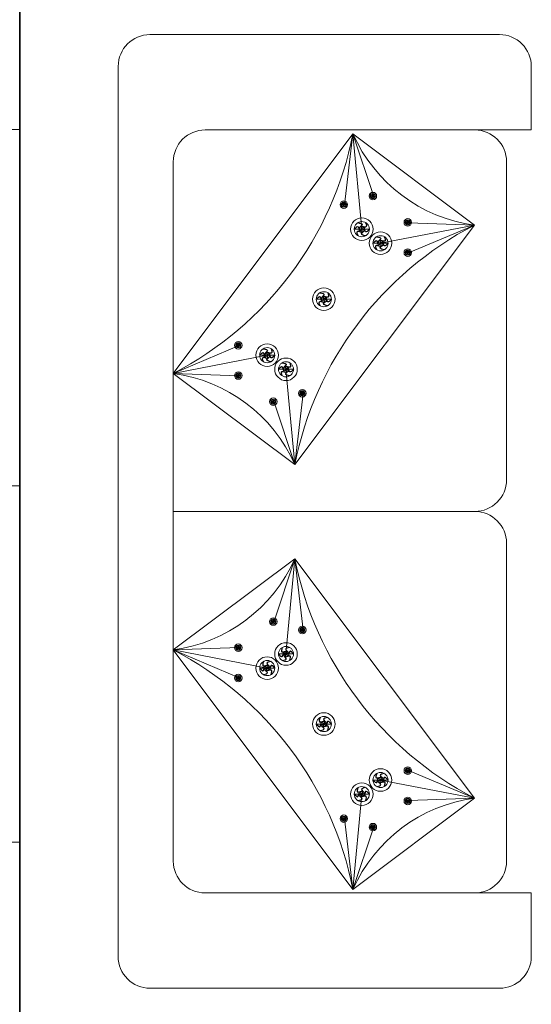
# Model space of a CAD drawing. Units: inches. Extents: x -61 to 1599, y -1316 to 257.
# Tile 164 of 204: x 1098 to 1130, y -901 to -839. Entities that reach past the tile are written whole.
import ezdxf

# ---------------------------------------------------------------- set-up
doc = ezdxf.new("R2010")
doc.units = ezdxf.units.IN
doc.header["$MEASUREMENT"] = 0
doc.layers.add('FUR', color=83, linetype='Continuous')
for name, color, linetype, lineweight in [('FURNITURE', 83, 'Continuous', 18), ('WALLS', 4, 'Continuous', 35), ('WINDOWS', 220, 'Continuous', 18)]:
    doc.layers.add(name, color=color, linetype=linetype, lineweight=lineweight)

# ---------------------------------------------------------------- blocks, each defined once
blk = doc.blocks.new('WIN-45IN')
for p, q in [((0, 44.83), (6, 44.83)), ((0, 0), (6, 0))]:
    blk.add_line(p, q)
for points in [[(6, 44.83), (3, 44.83), (3, 22.415), (6, 22.415)], [(3, 22.415), (0, 22.415), (0, 0), (3, 0)]]:
    blk.add_lwpolyline(points, close=True)
blk = doc.blocks.new('*U160')
at = {"layer": 'FUR'}
blk.add_open_spline([(0.005, 0.08), (-0.03, 0.048), (-0.098, -0.015), (0.075, -0.018), (0.024, -0.063), (0.005, -0.08)], degree=3, knots=[0, 0, 0, 0, 0.0954578, 0.1898773, 0.2470677, 0.2470677, 0.2470677, 0.2470677], dxfattribs=at)
blk = doc.blocks.new('*U161')
at = {"layer": 'FUR', "transparency": 16777216}
for p, rotation in [((222.173, -79.977), 60), ((222.312, -79.968), 300), ((222.178, -80.056), 120), ((222.25, -80.092), 180), ((222.317, -80.048), 240)]:
    blk.add_blockref('*U160', p, dxfattribs=dict(at, rotation=rotation))
blk.add_blockref('*U160', (222.24, -79.932), dxfattribs=at)
blk = doc.blocks.new('*U172')
at = {"layer": 'FUR'}
blk.add_open_spline([(0.005, 0.08), (-0.03, 0.048), (-0.098, -0.015), (0.075, -0.018), (0.024, -0.063), (0.005, -0.08)], degree=3, knots=[0, 0, 0, 0, 0.0954578, 0.1898773, 0.2470677, 0.2470677, 0.2470677, 0.2470677], dxfattribs=at)
blk = doc.blocks.new('*U173')
at = {"layer": 'FUR', "transparency": 16777216}
for p, rotation in [((222.173, -79.977), 60), ((222.312, -79.968), 300), ((222.178, -80.056), 120), ((222.25, -80.092), 180), ((222.317, -80.048), 240)]:
    blk.add_blockref('*U172', p, dxfattribs=dict(at, rotation=rotation))
blk.add_blockref('*U172', (222.24, -79.932), dxfattribs=at)
blk = doc.blocks.new('*U186')
at = {"layer": 'FUR'}
blk.add_open_spline([(0.005, 0.08), (-0.03, 0.048), (-0.098, -0.015), (0.075, -0.018), (0.024, -0.063), (0.005, -0.08)], degree=3, knots=[0, 0, 0, 0, 0.0954578, 0.1898773, 0.2470677, 0.2470677, 0.2470677, 0.2470677], dxfattribs=at)
blk = doc.blocks.new('*U187')
at = {"layer": 'FUR', "transparency": 16777216}
for p, rotation in [((222.173, -79.977), 60), ((222.312, -79.968), 300), ((222.178, -80.056), 120), ((222.25, -80.092), 180), ((222.317, -80.048), 240)]:
    blk.add_blockref('*U186', p, dxfattribs=dict(at, rotation=rotation))
blk.add_blockref('*U186', (222.24, -79.932), dxfattribs=at)
blk = doc.blocks.new('*U198')
at = {"layer": 'FUR'}
blk.add_open_spline([(0.005, 0.08), (-0.03, 0.048), (-0.098, -0.015), (0.075, -0.018), (0.024, -0.063), (0.005, -0.08)], degree=3, knots=[0, 0, 0, 0, 0.0954578, 0.1898773, 0.2470677, 0.2470677, 0.2470677, 0.2470677], dxfattribs=at)
blk = doc.blocks.new('*U199')
at = {"layer": 'FUR', "transparency": 16777216}
for p, rotation in [((222.173, -79.977), 60), ((222.312, -79.968), 300), ((222.178, -80.056), 120), ((222.25, -80.092), 180), ((222.317, -80.048), 240)]:
    blk.add_blockref('*U198', p, dxfattribs=dict(at, rotation=rotation))
blk.add_blockref('*U198', (222.24, -79.932), dxfattribs=at)
blk = doc.blocks.new('*U184')
at = {"layer": 'FUR'}
blk.add_open_spline([(0.015, 0.238), (-0.088, 0.143), (-0.292, -0.045), (0.224, -0.053), (0.072, -0.187), (0.015, -0.238)], degree=3, knots=[0, 0, 0, 0, 0.2846533, 0.5662105, 0.736751, 0.736751, 0.736751, 0.736751], dxfattribs=at)
blk = doc.blocks.new('*U159')
at = {"layer": 'FUR', "transparency": 16777216}
for p, rotation in [((662.517, -238.489), 60), ((662.929, -238.463), 300), ((662.944, -238.702), 240), ((662.531, -238.727), 120), ((662.745, -238.833), 180)]:
    blk.add_blockref('*U184', p, dxfattribs=dict(at, rotation=rotation))
blk.add_blockref('*U184', (662.716, -238.357), dxfattribs=at)
blk = doc.blocks.new('*U210')
at = {"layer": 'FUR'}
blk.add_open_spline([(0.015, 0.238), (-0.088, 0.143), (-0.292, -0.045), (0.224, -0.053), (0.072, -0.187), (0.015, -0.238)], degree=3, knots=[0, 0, 0, 0, 0.2846533, 0.5662105, 0.736751, 0.736751, 0.736751, 0.736751], dxfattribs=at)
blk = doc.blocks.new('*U185')
at = {"layer": 'FUR', "transparency": 16777216}
for p, rotation in [((662.517, -238.489), 60), ((662.929, -238.463), 300), ((662.944, -238.702), 240), ((662.531, -238.727), 120), ((662.745, -238.833), 180)]:
    blk.add_blockref('*U210', p, dxfattribs=dict(at, rotation=rotation))
blk.add_blockref('*U210', (662.716, -238.357), dxfattribs=at)
blk = doc.blocks.new('*U174')
at = {"layer": 'FUR'}
blk.add_open_spline([(0.005, 0.08), (-0.03, 0.048), (-0.098, -0.015), (0.075, -0.018), (0.024, -0.063), (0.005, -0.08)], degree=3, knots=[0, 0, 0, 0, 0.0954578, 0.1898773, 0.2470677, 0.2470677, 0.2470677, 0.2470677], dxfattribs=at)
blk = doc.blocks.new('*U175')
at = {"layer": 'FUR', "transparency": 16777216}
for p, rotation in [((222.173, -79.977), 60), ((222.312, -79.968), 300), ((222.178, -80.056), 120), ((222.25, -80.092), 180), ((222.317, -80.048), 240)]:
    blk.add_blockref('*U174', p, dxfattribs=dict(at, rotation=rotation))
blk.add_blockref('*U174', (222.24, -79.932), dxfattribs=at)
blk = doc.blocks.new('*U200')
at = {"layer": 'FUR'}
blk.add_open_spline([(0.005, 0.08), (-0.03, 0.048), (-0.098, -0.015), (0.075, -0.018), (0.024, -0.063), (0.005, -0.08)], degree=3, knots=[0, 0, 0, 0, 0.0954578, 0.1898773, 0.2470677, 0.2470677, 0.2470677, 0.2470677], dxfattribs=at)
blk = doc.blocks.new('*U201')
at = {"layer": 'FUR', "transparency": 16777216}
for p, rotation in [((222.173, -79.977), 60), ((222.312, -79.968), 300), ((222.178, -80.056), 120), ((222.25, -80.092), 180), ((222.317, -80.048), 240)]:
    blk.add_blockref('*U200', p, dxfattribs=dict(at, rotation=rotation))
blk.add_blockref('*U200', (222.24, -79.932), dxfattribs=at)
blk = doc.blocks.new('*U168')
at = {"layer": 'FUR'}
blk.add_open_spline([(0.015, 0.238), (-0.088, 0.143), (-0.292, -0.045), (0.224, -0.053), (0.072, -0.187), (0.015, -0.238)], degree=3, knots=[0, 0, 0, 0, 0.2846533, 0.5662105, 0.736751, 0.736751, 0.736751, 0.736751], dxfattribs=at)
blk = doc.blocks.new('*U169')
at = {"layer": 'FUR', "transparency": 16777216}
for p, rotation in [((662.517, -238.489), 60), ((662.929, -238.463), 300), ((662.944, -238.702), 240), ((662.531, -238.727), 120), ((662.745, -238.833), 180)]:
    blk.add_blockref('*U168', p, dxfattribs=dict(at, rotation=rotation))
blk.add_blockref('*U168', (662.716, -238.357), dxfattribs=at)
blk = doc.blocks.new('*U194')
at = {"layer": 'FUR'}
blk.add_open_spline([(0.015, 0.238), (-0.088, 0.143), (-0.292, -0.045), (0.224, -0.053), (0.072, -0.187), (0.015, -0.238)], degree=3, knots=[0, 0, 0, 0, 0.2846533, 0.5662105, 0.736751, 0.736751, 0.736751, 0.736751], dxfattribs=at)
blk = doc.blocks.new('*U195')
at = {"layer": 'FUR', "transparency": 16777216}
for p, rotation in [((662.517, -238.489), 60), ((662.929, -238.463), 300), ((662.944, -238.702), 240), ((662.531, -238.727), 120), ((662.745, -238.833), 180)]:
    blk.add_blockref('*U194', p, dxfattribs=dict(at, rotation=rotation))
blk.add_blockref('*U194', (662.716, -238.357), dxfattribs=at)
blk = doc.blocks.new('*U176')
at = {"layer": 'FUR'}
blk.add_open_spline([(0.005, 0.08), (-0.03, 0.048), (-0.098, -0.015), (0.075, -0.018), (0.024, -0.063), (0.005, -0.08)], degree=3, knots=[0, 0, 0, 0, 0.0954578, 0.1898773, 0.2470677, 0.2470677, 0.2470677, 0.2470677], dxfattribs=at)
blk = doc.blocks.new('*U177')
at = {"layer": 'FUR', "transparency": 16777216}
for p, rotation in [((222.173, -79.977), 60), ((222.312, -79.968), 300), ((222.178, -80.056), 120), ((222.25, -80.092), 180), ((222.317, -80.048), 240)]:
    blk.add_blockref('*U176', p, dxfattribs=dict(at, rotation=rotation))
blk.add_blockref('*U176', (222.24, -79.932), dxfattribs=at)
blk = doc.blocks.new('*U202')
at = {"layer": 'FUR'}
blk.add_open_spline([(0.005, 0.08), (-0.03, 0.048), (-0.098, -0.015), (0.075, -0.018), (0.024, -0.063), (0.005, -0.08)], degree=3, knots=[0, 0, 0, 0, 0.0954578, 0.1898773, 0.2470677, 0.2470677, 0.2470677, 0.2470677], dxfattribs=at)
blk = doc.blocks.new('*U203')
at = {"layer": 'FUR', "transparency": 16777216}
for p, rotation in [((222.173, -79.977), 60), ((222.312, -79.968), 300), ((222.178, -80.056), 120), ((222.25, -80.092), 180), ((222.317, -80.048), 240)]:
    blk.add_blockref('*U202', p, dxfattribs=dict(at, rotation=rotation))
blk.add_blockref('*U202', (222.24, -79.932), dxfattribs=at)
blk = doc.blocks.new('*U170')
at = {"layer": 'FUR'}
blk.add_open_spline([(0.015, 0.238), (-0.088, 0.143), (-0.292, -0.045), (0.224, -0.053), (0.072, -0.187), (0.015, -0.238)], degree=3, knots=[0, 0, 0, 0, 0.2846533, 0.5662105, 0.736751, 0.736751, 0.736751, 0.736751], dxfattribs=at)
blk = doc.blocks.new('*U171')
at = {"layer": 'FUR', "transparency": 16777216}
for p, rotation in [((662.517, -238.489), 60), ((662.929, -238.463), 300), ((662.944, -238.702), 240), ((662.531, -238.727), 120), ((662.745, -238.833), 180)]:
    blk.add_blockref('*U170', p, dxfattribs=dict(at, rotation=rotation))
blk.add_blockref('*U170', (662.716, -238.357), dxfattribs=at)
blk = doc.blocks.new('*U196')
at = {"layer": 'FUR'}
blk.add_open_spline([(0.015, 0.238), (-0.088, 0.143), (-0.292, -0.045), (0.224, -0.053), (0.072, -0.187), (0.015, -0.238)], degree=3, knots=[0, 0, 0, 0, 0.2846533, 0.5662105, 0.736751, 0.736751, 0.736751, 0.736751], dxfattribs=at)
blk = doc.blocks.new('*U197')
at = {"layer": 'FUR', "transparency": 16777216}
for p, rotation in [((662.517, -238.489), 60), ((662.929, -238.463), 300), ((662.944, -238.702), 240), ((662.531, -238.727), 120), ((662.745, -238.833), 180)]:
    blk.add_blockref('*U196', p, dxfattribs=dict(at, rotation=rotation))
blk.add_blockref('*U196', (662.716, -238.357), dxfattribs=at)
blk = doc.blocks.new('*U164')
at = {"layer": 'FUR'}
blk.add_open_spline([(0.005, 0.08), (-0.03, 0.048), (-0.098, -0.015), (0.075, -0.018), (0.024, -0.063), (0.005, -0.08)], degree=3, knots=[0, 0, 0, 0, 0.0954578, 0.1898773, 0.2470677, 0.2470677, 0.2470677, 0.2470677], dxfattribs=at)
blk = doc.blocks.new('*U165')
at = {"layer": 'FUR', "transparency": 16777216}
for p, rotation in [((222.173, -79.977), 60), ((222.312, -79.968), 300), ((222.178, -80.056), 120), ((222.25, -80.092), 180), ((222.317, -80.048), 240)]:
    blk.add_blockref('*U164', p, dxfattribs=dict(at, rotation=rotation))
blk.add_blockref('*U164', (222.24, -79.932), dxfattribs=at)
blk = doc.blocks.new('*U190')
at = {"layer": 'FUR'}
blk.add_open_spline([(0.005, 0.08), (-0.03, 0.048), (-0.098, -0.015), (0.075, -0.018), (0.024, -0.063), (0.005, -0.08)], degree=3, knots=[0, 0, 0, 0, 0.0954578, 0.1898773, 0.2470677, 0.2470677, 0.2470677, 0.2470677], dxfattribs=at)
blk = doc.blocks.new('*U191')
at = {"layer": 'FUR', "transparency": 16777216}
for p, rotation in [((222.173, -79.977), 60), ((222.312, -79.968), 300), ((222.178, -80.056), 120), ((222.25, -80.092), 180), ((222.317, -80.048), 240)]:
    blk.add_blockref('*U190', p, dxfattribs=dict(at, rotation=rotation))
blk.add_blockref('*U190', (222.24, -79.932), dxfattribs=at)
blk = doc.blocks.new('*U183')
at = {"layer": 'FUR'}
blk.add_open_spline([(0.015, 0.238), (-0.088, 0.143), (-0.292, -0.045), (0.224, -0.053), (0.072, -0.187), (0.015, -0.238)], degree=3, knots=[0, 0, 0, 0, 0.2846533, 0.5662105, 0.736751, 0.736751, 0.736751, 0.736751], dxfattribs=at)
blk = doc.blocks.new('*U162')
at = {"layer": 'FUR', "transparency": 16777216}
for p, rotation in [((662.517, -238.489), 60), ((662.929, -238.463), 300), ((662.944, -238.702), 240), ((662.531, -238.727), 120), ((662.745, -238.833), 180)]:
    blk.add_blockref('*U183', p, dxfattribs=dict(at, rotation=rotation))
blk.add_blockref('*U183', (662.716, -238.357), dxfattribs=at)
blk = doc.blocks.new('*U209')
at = {"layer": 'FUR'}
blk.add_open_spline([(0.015, 0.238), (-0.088, 0.143), (-0.292, -0.045), (0.224, -0.053), (0.072, -0.187), (0.015, -0.238)], degree=3, knots=[0, 0, 0, 0, 0.2846533, 0.5662105, 0.736751, 0.736751, 0.736751, 0.736751], dxfattribs=at)
blk = doc.blocks.new('*U188')
at = {"layer": 'FUR', "transparency": 16777216}
for p, rotation in [((662.517, -238.489), 60), ((662.929, -238.463), 300), ((662.944, -238.702), 240), ((662.531, -238.727), 120), ((662.745, -238.833), 180)]:
    blk.add_blockref('*U209', p, dxfattribs=dict(at, rotation=rotation))
blk.add_blockref('*U209', (662.716, -238.357), dxfattribs=at)
blk = doc.blocks.new('*U182')
at = {"layer": 'FUR'}
blk.add_open_spline([(0.005, 0.08), (-0.03, 0.048), (-0.098, -0.015), (0.075, -0.018), (0.024, -0.063), (0.005, -0.08)], degree=3, knots=[0, 0, 0, 0, 0.0954578, 0.1898773, 0.2470677, 0.2470677, 0.2470677, 0.2470677], dxfattribs=at)
blk = doc.blocks.new('*U163')
at = {"layer": 'FUR', "transparency": 16777216}
for p, rotation in [((222.173, -79.977), 60), ((222.312, -79.968), 300), ((222.178, -80.056), 120), ((222.25, -80.092), 180), ((222.317, -80.048), 240)]:
    blk.add_blockref('*U182', p, dxfattribs=dict(at, rotation=rotation))
blk.add_blockref('*U182', (222.24, -79.932), dxfattribs=at)
blk = doc.blocks.new('*U208')
at = {"layer": 'FUR'}
blk.add_open_spline([(0.005, 0.08), (-0.03, 0.048), (-0.098, -0.015), (0.075, -0.018), (0.024, -0.063), (0.005, -0.08)], degree=3, knots=[0, 0, 0, 0, 0.0954578, 0.1898773, 0.2470677, 0.2470677, 0.2470677, 0.2470677], dxfattribs=at)
blk = doc.blocks.new('*U189')
at = {"layer": 'FUR', "transparency": 16777216}
for p, rotation in [((222.173, -79.977), 60), ((222.312, -79.968), 300), ((222.178, -80.056), 120), ((222.25, -80.092), 180), ((222.317, -80.048), 240)]:
    blk.add_blockref('*U208', p, dxfattribs=dict(at, rotation=rotation))
blk.add_blockref('*U208', (222.24, -79.932), dxfattribs=at)
blk = doc.blocks.new('*U166')
at = {"layer": 'FUR'}
blk.add_open_spline([(0.015, 0.238), (-0.088, 0.143), (-0.292, -0.045), (0.224, -0.053), (0.072, -0.187), (0.015, -0.238)], degree=3, knots=[0, 0, 0, 0, 0.2846533, 0.5662105, 0.736751, 0.736751, 0.736751, 0.736751], dxfattribs=at)
blk = doc.blocks.new('*U167')
at = {"layer": 'FUR', "transparency": 16777216}
for p, rotation in [((662.517, -238.489), 60), ((662.929, -238.463), 300), ((662.944, -238.702), 240), ((662.531, -238.727), 120), ((662.745, -238.833), 180)]:
    blk.add_blockref('*U166', p, dxfattribs=dict(at, rotation=rotation))
blk.add_blockref('*U166', (662.716, -238.357), dxfattribs=at)
blk = doc.blocks.new('*U192')
at = {"layer": 'FUR'}
blk.add_open_spline([(0.015, 0.238), (-0.088, 0.143), (-0.292, -0.045), (0.224, -0.053), (0.072, -0.187), (0.015, -0.238)], degree=3, knots=[0, 0, 0, 0, 0.2846533, 0.5662105, 0.736751, 0.736751, 0.736751, 0.736751], dxfattribs=at)
blk = doc.blocks.new('*U193')
at = {"layer": 'FUR', "transparency": 16777216}
for p, rotation in [((662.517, -238.489), 60), ((662.929, -238.463), 300), ((662.944, -238.702), 240), ((662.531, -238.727), 120), ((662.745, -238.833), 180)]:
    blk.add_blockref('*U192', p, dxfattribs=dict(at, rotation=rotation))
blk.add_blockref('*U192', (662.716, -238.357), dxfattribs=at)
blk = doc.blocks.new('*U178')
at = {"layer": 'FUR'}
blk.add_open_spline([(0.005, 0.08), (-0.03, 0.048), (-0.098, -0.015), (0.075, -0.018), (0.024, -0.063), (0.005, -0.08)], degree=3, knots=[0, 0, 0, 0, 0.0954578, 0.1898773, 0.2470677, 0.2470677, 0.2470677, 0.2470677], dxfattribs=at)
blk = doc.blocks.new('*U179')
at = {"layer": 'FUR', "transparency": 16777216}
for p, rotation in [((222.173, -79.977), 60), ((222.312, -79.968), 300), ((222.178, -80.056), 120), ((222.25, -80.092), 180), ((222.317, -80.048), 240)]:
    blk.add_blockref('*U178', p, dxfattribs=dict(at, rotation=rotation))
blk.add_blockref('*U178', (222.24, -79.932), dxfattribs=at)
blk = doc.blocks.new('*U180')
at = {"layer": 'FUR'}
blk.add_open_spline([(0.005, 0.08), (-0.03, 0.048), (-0.098, -0.015), (0.075, -0.018), (0.024, -0.063), (0.005, -0.08)], degree=3, knots=[0, 0, 0, 0, 0.0954578, 0.1898773, 0.2470677, 0.2470677, 0.2470677, 0.2470677], dxfattribs=at)
blk = doc.blocks.new('*U181')
at = {"layer": 'FUR', "transparency": 16777216}
for p, rotation in [((222.173, -79.977), 60), ((222.312, -79.968), 300), ((222.178, -80.056), 120), ((222.25, -80.092), 180), ((222.317, -80.048), 240)]:
    blk.add_blockref('*U180', p, dxfattribs=dict(at, rotation=rotation))
blk.add_blockref('*U180', (222.24, -79.932), dxfattribs=at)
blk = doc.blocks.new('*U204')
at = {"layer": 'FUR'}
blk.add_open_spline([(0.005, 0.08), (-0.03, 0.048), (-0.098, -0.015), (0.075, -0.018), (0.024, -0.063), (0.005, -0.08)], degree=3, knots=[0, 0, 0, 0, 0.0954578, 0.1898773, 0.2470677, 0.2470677, 0.2470677, 0.2470677], dxfattribs=at)
blk = doc.blocks.new('*U205')
at = {"layer": 'FUR', "transparency": 16777216}
for p, rotation in [((222.173, -79.977), 60), ((222.312, -79.968), 300), ((222.178, -80.056), 120), ((222.25, -80.092), 180), ((222.317, -80.048), 240)]:
    blk.add_blockref('*U204', p, dxfattribs=dict(at, rotation=rotation))
blk.add_blockref('*U204', (222.24, -79.932), dxfattribs=at)
blk = doc.blocks.new('*U206')
at = {"layer": 'FUR'}
blk.add_open_spline([(0.005, 0.08), (-0.03, 0.048), (-0.098, -0.015), (0.075, -0.018), (0.024, -0.063), (0.005, -0.08)], degree=3, knots=[0, 0, 0, 0, 0.0954578, 0.1898773, 0.2470677, 0.2470677, 0.2470677, 0.2470677], dxfattribs=at)
blk = doc.blocks.new('*U207')
at = {"layer": 'FUR', "transparency": 16777216}
for p, rotation in [((222.173, -79.977), 60), ((222.312, -79.968), 300), ((222.178, -80.056), 120), ((222.25, -80.092), 180), ((222.317, -80.048), 240)]:
    blk.add_blockref('*U206', p, dxfattribs=dict(at, rotation=rotation))
blk.add_blockref('*U206', (222.24, -79.932), dxfattribs=at)
blk = doc.blocks.new('SOFA-LOVESEAT')
for p, q in [((22.442, 54), (5.47, 54)), ((22.442, 54), (26, 54)), ((14.776, 53.751), (14.253, 49.285)), ((14.776, 53.751), (15.332, 47.757)), ((14.776, 53.751), (16.081, 49.817)), ((3.47, 8), (3.47, 52)), ((24.442, 52), (24.442, 32)), ((16.029, 49.837), (15.869, 49.837)), ((16.029, 49.837), (16.189, 49.837)), ((14.201, 49.305), (14.041, 49.305)), ((14.201, 49.305), (14.36, 49.305)), ((15.332, 47.757), (14.855, 47.757)), ((15.332, 47.757), (15.808, 47.757)), ((22.422, 48.013), (16.511, 46.872)), ((18.228, 48.187), (18.068, 48.187)), ((18.228, 48.187), (18.388, 48.187)), ((22.422, 48.013), (18.28, 48.167)), ((22.422, 48.013), (18.28, 46.263)), ((16.511, 46.872), (16.035, 46.872)), ((16.511, 46.872), (16.988, 46.872)), ((18.228, 46.282), (18.068, 46.282)), ((18.228, 46.282), (18.388, 46.282)), ((12.946, 43.35), (12.47, 43.35)), ((12.946, 43.35), (13.423, 43.35)), ((3.47, 38.686), (7.612, 40.436)), ((7.56, 40.455), (7.4, 40.455)), ((7.56, 40.455), (7.719, 40.455)), ((3.47, 38.686), (9.381, 39.828)), ((9.381, 39.828), (8.904, 39.828)), ((9.381, 39.828), (9.857, 39.828)), ((3.47, 38.686), (7.612, 38.532)), ((7.56, 38.551), (7.4, 38.551)), ((7.56, 38.551), (7.719, 38.551)), ((10.561, 38.942), (10.084, 38.942)), ((11.116, 32.948), (10.561, 38.942)), ((10.561, 38.942), (11.037, 38.942)), ((11.116, 32.948), (11.639, 37.414)), ((11.587, 37.433), (11.427, 37.433)), ((11.587, 37.433), (11.747, 37.433)), ((9.759, 36.901), (9.599, 36.901)), ((9.759, 36.901), (9.918, 36.901)), ((11.116, 32.948), (9.811, 36.882)), ((22.442, 30), (3.47, 30)), ((22.442, 30), (22.442, 30)), ((24.442, 8), (24.442, 28)), ((11.116, 27.026), (9.811, 23.092)), ((11.116, 27.026), (10.561, 21.032)), ((11.116, 27.026), (11.639, 22.56)), ((9.759, 23.073), (9.599, 23.073)), ((9.759, 23.073), (9.918, 23.073)), ((11.587, 22.541), (11.427, 22.541)), ((11.587, 22.541), (11.747, 22.541)), ((3.47, 21.288), (7.612, 21.442)), ((3.47, 21.288), (9.381, 20.146)), ((3.47, 21.288), (7.612, 19.538)), ((7.56, 21.423), (7.4, 21.423)), ((7.56, 21.423), (7.719, 21.423)), ((10.561, 21.032), (10.084, 21.032)), ((10.561, 21.032), (11.037, 21.032)), ((9.381, 20.146), (8.904, 20.146)), ((9.381, 20.146), (9.857, 20.146)), ((7.56, 19.518), (7.4, 19.518)), ((7.56, 19.518), (7.719, 19.518)), ((12.946, 16.624), (12.47, 16.624)), ((12.946, 16.624), (13.423, 16.624)), ((18.228, 13.691), (18.068, 13.691)), ((18.228, 13.691), (18.388, 13.691)), ((22.422, 11.961), (18.28, 13.711)), ((16.511, 13.102), (16.035, 13.102)), ((22.422, 11.961), (16.511, 13.102)), ((16.511, 13.102), (16.988, 13.102)), ((14.776, 6.223), (15.332, 12.217)), ((15.332, 12.217), (14.855, 12.217)), ((15.332, 12.217), (15.808, 12.217)), ((18.228, 11.787), (18.068, 11.787)), ((18.228, 11.787), (18.388, 11.787)), ((22.422, 11.961), (18.28, 11.807)), ((14.201, 10.669), (14.041, 10.669)), ((14.201, 10.669), (14.36, 10.669)), ((14.776, 6.223), (14.253, 10.689)), ((14.776, 6.223), (16.081, 10.156)), ((16.029, 10.137), (15.869, 10.137)), ((16.029, 10.137), (16.189, 10.137)), ((22.442, 6), (5.47, 6)), ((22.442, 6), (26, 6))]:
    blk.add_line(p, q)
blk.add_lwpolyline([(26, 6), (26, 2, -0.414214), (24, 0), (2, 0, -0.414214), (0, 2), (0, 58, -0.414213), (2, 60), (24, 60, -0.414214), (26, 58), (26, 54)], format="xyb")
for points in [[(11.116, 32.948), (22.422, 48.013), (14.776, 53.751), (3.47, 38.686)], [(11.116, 27.026), (22.422, 11.961), (14.776, 6.223), (3.47, 21.288)]]:
    blk.add_lwpolyline(points, close=True)
for centre, radius in [((16.029, 49.837), 0.238), ((16.029, 49.837), 0.16), ((14.201, 49.305), 0.238), ((14.201, 49.305), 0.16), ((15.332, 47.757), 0.71), ((18.228, 48.187), 0.238), ((18.228, 48.187), 0.16), ((15.332, 47.757), 0.476), ((16.511, 46.872), 0.71), ((16.511, 46.872), 0.476), ((18.228, 46.282), 0.238), ((18.228, 46.282), 0.16), ((12.946, 43.35), 0.71), ((12.946, 43.35), 0.476), ((7.56, 40.455), 0.238), ((7.56, 40.455), 0.16), ((9.381, 39.828), 0.71), ((9.381, 39.828), 0.476), ((10.561, 38.942), 0.71), ((10.561, 38.942), 0.476), ((7.56, 38.551), 0.238), ((7.56, 38.551), 0.16), ((11.587, 37.433), 0.238), ((11.587, 37.433), 0.16), ((9.759, 36.901), 0.238), ((9.759, 36.901), 0.16), ((9.759, 23.073), 0.238), ((9.759, 23.073), 0.16), ((11.587, 22.541), 0.238), ((11.587, 22.541), 0.16), ((10.561, 21.032), 0.71), ((7.56, 21.423), 0.238), ((7.56, 21.423), 0.16), ((10.561, 21.032), 0.476), ((9.381, 20.146), 0.71), ((9.381, 20.146), 0.476), ((7.56, 19.518), 0.238), ((7.56, 19.518), 0.16), ((12.946, 16.624), 0.71), ((12.946, 16.624), 0.476), ((16.511, 13.102), 0.71), ((18.228, 13.691), 0.238), ((18.228, 13.691), 0.16), ((16.511, 13.102), 0.476), ((15.332, 12.217), 0.71), ((15.332, 12.217), 0.476), ((18.228, 11.787), 0.238), ((18.228, 11.787), 0.16), ((14.201, 10.669), 0.238), ((14.201, 10.669), 0.16), ((16.029, 10.137), 0.238), ((16.029, 10.137), 0.16)]:
    blk.add_circle(centre, radius)
for centre, radius, start, end in [((5.47, 52), 2, 90, 180.00002), ((22.442, 52), 2, 0, 90), ((-6.541, 57.974), 21.731, 297.43166, 348.79559), ((23.745, 57.74), 9.816, 203.97425, 262.253), ((32.433, 28.726), 21.731, 117.43166, 168.79559), ((2.147, 28.96), 9.816, 23.97425, 82.253), ((22.442, 32), 2, 270, 0), ((22.442, 28), 2, 0, 90), ((2.147, 31.014), 9.816, 277.74703, 336.02578), ((32.433, 31.248), 21.731, 191.20444, 242.56837), ((-6.541, 2), 21.731, 11.20444, 62.56837), ((23.745, 2.234), 9.816, 97.74703, 156.02578), ((5.47, 8), 2, 180.00002, 270), ((22.442, 8), 2, 270, 0)]:
    blk.add_arc(centre, radius, start, end)
at = {"xscale": -1, "rotation": 90.00003000000098}
for name, p in [('*U189', (-63.984, 272.082)), ('*U191', (-65.812, 271.55)), ('*U205', (-61.785, 270.431)), ('*U188', (-223.264, 710.487)), ('*U193', (-222.084, 709.602)), ('*U207', (-61.785, 268.527)), ('*U197', (-225.649, 706.08)), ('*U187', (-72.453, 262.7)), ('*U185', (-229.215, 702.558)), ('*U195', (-228.035, 701.672)), ('*U199', (-72.453, 260.796)), ('*U203', (-68.426, 259.678)), ('*U201', (-70.254, 259.146))]:
    blk.add_blockref(name, p, dxfattribs=at)
at = {"rotation": 90}
for name, p in [('*U175', (-70.254, -199.172)), ('*U177', (-68.425, -199.704)), ('*U173', (-72.453, -200.822)), ('*U169', (-228.034, -641.698)), ('*U159', (-229.214, -642.584)), ('*U161', (-72.453, -202.727)), ('*U171', (-225.649, -646.106)), ('*U181', (-61.785, -208.554)), ('*U167', (-222.084, -649.628)), ('*U162', (-223.264, -650.513)), ('*U179', (-61.785, -210.458)), ('*U165', (-65.812, -211.576)), ('*U163', (-63.983, -212.108))]:
    blk.add_blockref(name, p, dxfattribs=at)

msp = doc.modelspace()

# ---------------------------------------------------------------- linework, layer by layer
at = {"layer": 'WALLS'}
msp.add_line((1097.7028, -939.169), (1097.7028, -783.169), dxfattribs=at)

# ---------------------------------------------------------------- block references
at = {"layer": 'FURNITURE'}
msp.add_blockref('SOFA-LOVESEAT', (1103.901, -899.5411), dxfattribs=at)
at = {"layer": 'WINDOWS'}
msp.add_blockref('WIN-45IN', (1091.703, -890.3441), dxfattribs=at)

doc.saveas('drawing.dxf')
